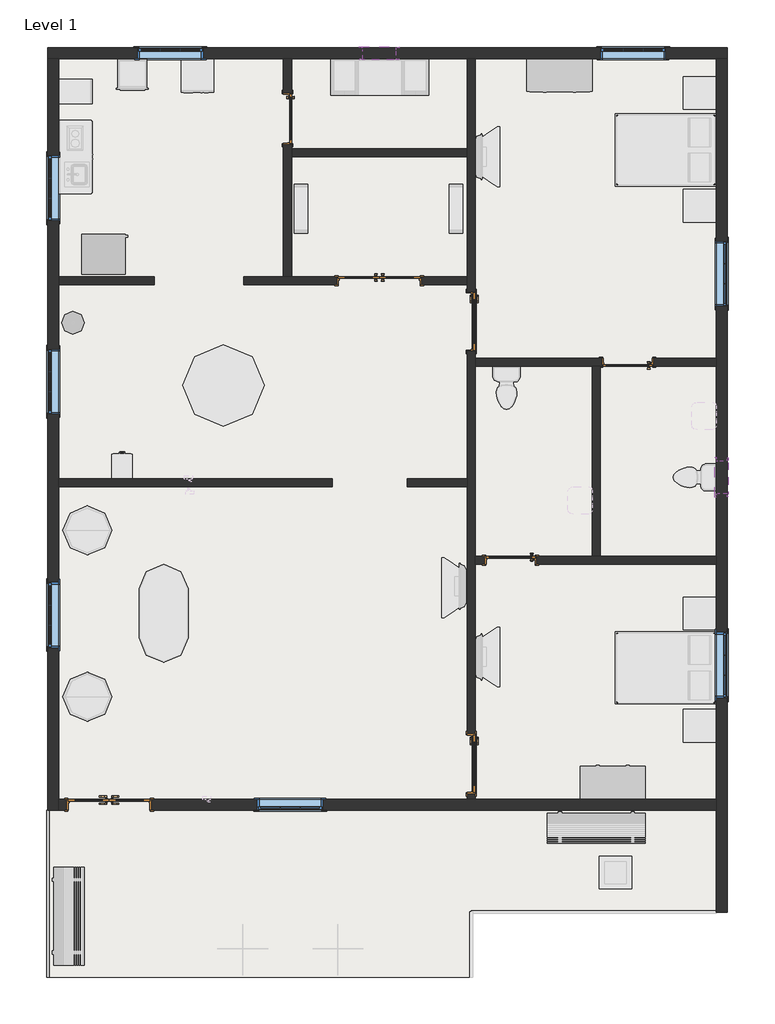
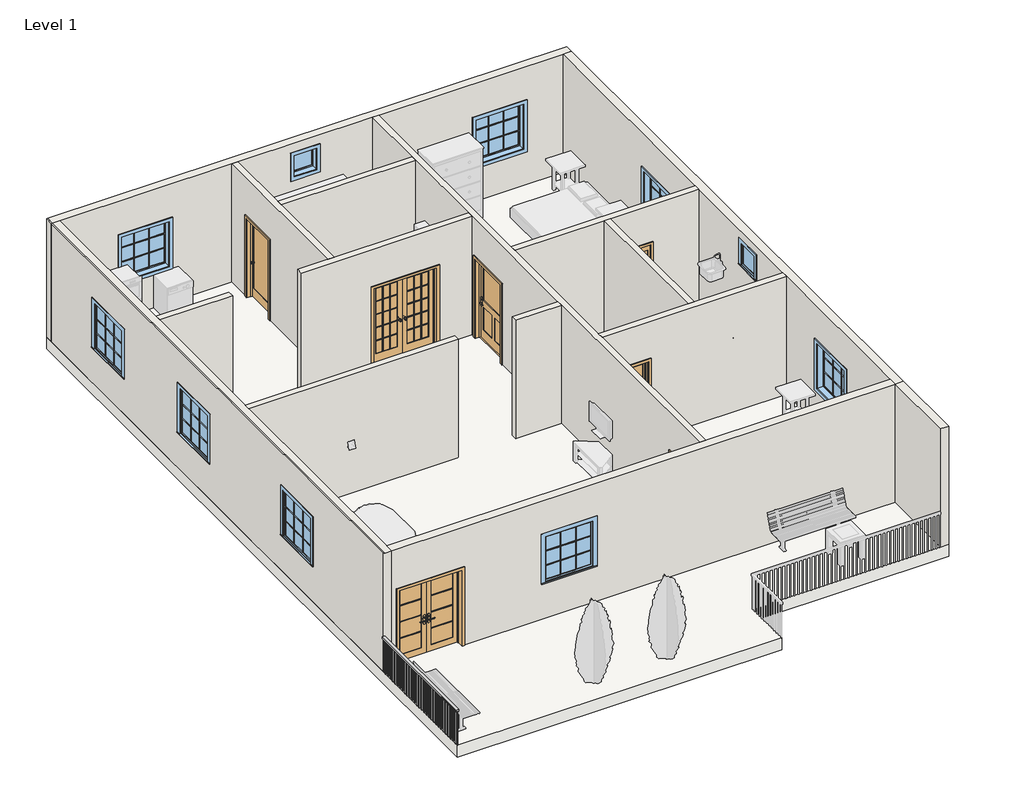
# One storey, part 1 of 2: 14 walls, 10 windows, 7 doors, 1 railing, 1 slab.
"""IFC4 building model written with IfcOpenShell, lengths in millimetres."""

from ifc_helpers import new_model, si_unit, frame, origin, origin_with_axes, place, context, project, spatial, polyline, outline, extrude, faceted_brep, transform, mapped, element, save
from components import door_f970b2d0, door_b03bd389, door_31a77bde, door_b28d7136, door_792ab218, window_791d807c, window_7418cbd4, window_e41d21a6

model = new_model("IFC4")

# Units and contexts
model_context = context("Model", 3, world=origin())
ifc_project = project(units=[si_unit("LENGTHUNIT", "METRE", prefix="MILLI")], contexts=[model_context])

# Site, building, storey
site = spatial("IfcSite", under=ifc_project)
building = spatial("IfcBuilding", under=site)
storey = spatial("IfcBuildingStorey", under=building, Name="Level 1", Elevation=0.0)

# Doors
placement = place(None, origin())
door_shape = door_f970b2d0(model_context)
element("IfcDoor", 1, ObjectType="30\" x 80\"", at=placement, inside=storey, context=model_context, shape_type="MappedRepresentation", body=[
    mapped(door_shape, transform((-7653.2898609, 8737.7801051, 0.0), x_axis=(0.0, 1.0, 0.0), y_axis=(-1.0, 0.0, 0.0), z_axis=(0.0, 0.0, 1.0))),
])
element("IfcDoor", 2, ObjectType="30\" x 80\"", at=placement, inside=storey, context=model_context, shape_type="MappedRepresentation", body=[
    mapped(door_shape, transform((-7653.2898609, 482.7801051, 0.0), x_axis=(0.0, 1.0, 0.0), y_axis=(-1.0, 0.0, 0.0), z_axis=(0.0, 0.0, 1.0))),
])
door_2_shape = door_b03bd389(model_context)
element("IfcDoor", 3, ObjectType="Door-Exterior-Double-Full Glass-Wood_Clad : 60\" x 80\"", at=placement, inside=storey, context=model_context, shape_type="MappedRepresentation", body=[
    mapped(door_2_shape, transform((-14412.8648609, -276.0448949, -76.2), x_axis=(1.0, 0.0, 0.0), y_axis=(0.0, 1.0, 0.0), z_axis=(0.0, 0.0, 1.0))),
])
door_3_shape = door_31a77bde(model_context)
element("IfcDoor", 4, ObjectType="Door-Interior-Double-Full Glass-Wood : 60\" x 80\"", at=placement, inside=storey, context=model_context, shape_type="MappedRepresentation", body=[
    mapped(door_3_shape, transform((-9370.9648609, 9502.9551051, 0.0), x_axis=(1.0, 0.0, 0.0), y_axis=(0.0, 1.0, 0.0), z_axis=(0.0, 0.0, 1.0))),
])
door_4_shape = door_b28d7136(model_context)
element("IfcDoor", 5, ObjectType="Door-Interior-Single-1_Panel-Wood : 12\" x 80\"", at=placement, inside=storey, context=model_context, shape_type="MappedRepresentation", body=[
    mapped(door_4_shape, transform((-4735.4648609, 7972.6051051, 0.0), x_axis=(-1.0, 0.0, 0.0), y_axis=(0.0, -1.0, 0.0), z_axis=(0.0, 0.0, 1.0))),
])
element("IfcDoor", 6, ObjectType="Door-Interior-Single-1_Panel-Wood : 12\" x 80\"", at=placement, inside=storey, context=model_context, shape_type="MappedRepresentation", body=[
    mapped(door_4_shape, transform((-11082.2898609, 12522.3801051, 0.0), x_axis=(0.0, -1.0, 0.0), y_axis=(1.0, 0.0, 0.0), z_axis=(0.0, 0.0, 1.0))),
])
door_5_shape = door_792ab218(model_context)
element("IfcDoor", 7, ObjectType="Door-Interior-Single-1_Panel-Wood : 12\" x 80\"", at=placement, inside=storey, context=model_context, shape_type="MappedRepresentation", body=[
    mapped(door_5_shape, transform((-6919.8648609, 4283.2551051, 0.0), x_axis=(-1.0, 0.0, 0.0), y_axis=(0.0, -1.0, 0.0), z_axis=(0.0, 0.0, 1.0))),
])

# Railing
element("IfcRailing", 8, ObjectType="Handrail - Rectangular", at=placement, inside=storey, context=model_context, shape_type="SweptSolid", body=[
    extrude(outline(polyline([(-15581.2648609, -380.8198949), (-15530.4648609, -380.8198949), (-15530.4648609, -3505.0198949), (-15581.2648609, -3505.0198949), (-15581.2648609, -380.8198949)])), frame((0.0, 0.0, 863.6), z_axis=(0.0, 0.0, 1.0), x_axis=(1.0, 0.0, 0.0)), (0.0, 0.0, 1.0), 50.8),
    extrude(outline(polyline([(-15565.3898609, -3419.2948949), (-15546.3398609, -3419.2948949), (-15546.3398609, -3438.3448949), (-15565.3898609, -3438.3448949), (-15565.3898609, -3419.2948949)])), origin_with_axes(), (0.0, 0.0, 1.0), 863.6),
    extrude(outline(polyline([(-15565.3898609, -3317.6948949), (-15546.3398609, -3317.6948949), (-15546.3398609, -3336.7448949), (-15565.3898609, -3336.7448949), (-15565.3898609, -3317.6948949)])), origin_with_axes(), (0.0, 0.0, 1.0), 863.6),
    extrude(outline(polyline([(-15565.3898609, -3216.0948949), (-15546.3398609, -3216.0948949), (-15546.3398609, -3235.1448949), (-15565.3898609, -3235.1448949), (-15565.3898609, -3216.0948949)])), origin_with_axes(), (0.0, 0.0, 1.0), 863.6),
    extrude(outline(polyline([(-15565.3898609, -3114.4948949), (-15546.3398609, -3114.4948949), (-15546.3398609, -3133.5448949), (-15565.3898609, -3133.5448949), (-15565.3898609, -3114.4948949)])), origin_with_axes(), (0.0, 0.0, 1.0), 863.6),
    extrude(outline(polyline([(-15565.3898609, -3012.8948949), (-15546.3398609, -3012.8948949), (-15546.3398609, -3031.9448949), (-15565.3898609, -3031.9448949), (-15565.3898609, -3012.8948949)])), origin_with_axes(), (0.0, 0.0, 1.0), 863.6),
    extrude(outline(polyline([(-15565.3898609, -2911.2948949), (-15546.3398609, -2911.2948949), (-15546.3398609, -2930.3448949), (-15565.3898609, -2930.3448949), (-15565.3898609, -2911.2948949)])), origin_with_axes(), (0.0, 0.0, 1.0), 863.6),
    extrude(outline(polyline([(-15565.3898609, -2809.6948949), (-15546.3398609, -2809.6948949), (-15546.3398609, -2828.7448949), (-15565.3898609, -2828.7448949), (-15565.3898609, -2809.6948949)])), origin_with_axes(), (0.0, 0.0, 1.0), 863.6),
    extrude(outline(polyline([(-15565.3898609, -2708.0948949), (-15546.3398609, -2708.0948949), (-15546.3398609, -2727.1448949), (-15565.3898609, -2727.1448949), (-15565.3898609, -2708.0948949)])), origin_with_axes(), (0.0, 0.0, 1.0), 863.6),
    extrude(outline(polyline([(-15565.3898609, -2606.4948949), (-15546.3398609, -2606.4948949), (-15546.3398609, -2625.5448949), (-15565.3898609, -2625.5448949), (-15565.3898609, -2606.4948949)])), origin_with_axes(), (0.0, 0.0, 1.0), 863.6),
    extrude(outline(polyline([(-15565.3898609, -2504.8948949), (-15546.3398609, -2504.8948949), (-15546.3398609, -2523.9448949), (-15565.3898609, -2523.9448949), (-15565.3898609, -2504.8948949)])), origin_with_axes(), (0.0, 0.0, 1.0), 863.6),
    extrude(outline(polyline([(-15565.3898609, -2403.2948949), (-15546.3398609, -2403.2948949), (-15546.3398609, -2422.3448949), (-15565.3898609, -2422.3448949), (-15565.3898609, -2403.2948949)])), origin_with_axes(), (0.0, 0.0, 1.0), 863.6),
    extrude(outline(polyline([(-15565.3898609, -2301.6948949), (-15546.3398609, -2301.6948949), (-15546.3398609, -2320.7448949), (-15565.3898609, -2320.7448949), (-15565.3898609, -2301.6948949)])), origin_with_axes(), (0.0, 0.0, 1.0), 863.6),
    extrude(outline(polyline([(-15565.3898609, -2200.0948949), (-15546.3398609, -2200.0948949), (-15546.3398609, -2219.1448949), (-15565.3898609, -2219.1448949), (-15565.3898609, -2200.0948949)])), origin_with_axes(), (0.0, 0.0, 1.0), 863.6),
    extrude(outline(polyline([(-15565.3898609, -2098.4948949), (-15546.3398609, -2098.4948949), (-15546.3398609, -2117.5448949), (-15565.3898609, -2117.5448949), (-15565.3898609, -2098.4948949)])), origin_with_axes(), (0.0, 0.0, 1.0), 863.6),
    extrude(outline(polyline([(-15565.3898609, -1996.8948949), (-15546.3398609, -1996.8948949), (-15546.3398609, -2015.9448949), (-15565.3898609, -2015.9448949), (-15565.3898609, -1996.8948949)])), origin_with_axes(), (0.0, 0.0, 1.0), 863.6),
    extrude(outline(polyline([(-15565.3898609, -1895.2948949), (-15546.3398609, -1895.2948949), (-15546.3398609, -1914.3448949), (-15565.3898609, -1914.3448949), (-15565.3898609, -1895.2948949)])), origin_with_axes(), (0.0, 0.0, 1.0), 863.6),
    extrude(outline(polyline([(-15565.3898609, -1793.6948949), (-15546.3398609, -1793.6948949), (-15546.3398609, -1812.7448949), (-15565.3898609, -1812.7448949), (-15565.3898609, -1793.6948949)])), origin_with_axes(), (0.0, 0.0, 1.0), 863.6),
    extrude(outline(polyline([(-15565.3898609, -1692.0948949), (-15546.3398609, -1692.0948949), (-15546.3398609, -1711.1448949), (-15565.3898609, -1711.1448949), (-15565.3898609, -1692.0948949)])), origin_with_axes(), (0.0, 0.0, 1.0), 863.6),
    extrude(outline(polyline([(-15565.3898609, -1590.4948949), (-15546.3398609, -1590.4948949), (-15546.3398609, -1609.5448949), (-15565.3898609, -1609.5448949), (-15565.3898609, -1590.4948949)])), origin_with_axes(), (0.0, 0.0, 1.0), 863.6),
    extrude(outline(polyline([(-15565.3898609, -1488.8948949), (-15546.3398609, -1488.8948949), (-15546.3398609, -1507.9448949), (-15565.3898609, -1507.9448949), (-15565.3898609, -1488.8948949)])), origin_with_axes(), (0.0, 0.0, 1.0), 863.6),
    extrude(outline(polyline([(-15565.3898609, -1387.2948949), (-15546.3398609, -1387.2948949), (-15546.3398609, -1406.3448949), (-15565.3898609, -1406.3448949), (-15565.3898609, -1387.2948949)])), origin_with_axes(), (0.0, 0.0, 1.0), 863.6),
    extrude(outline(polyline([(-15565.3898609, -1285.6948949), (-15546.3398609, -1285.6948949), (-15546.3398609, -1304.7448949), (-15565.3898609, -1304.7448949), (-15565.3898609, -1285.6948949)])), origin_with_axes(), (0.0, 0.0, 1.0), 863.6),
    extrude(outline(polyline([(-15565.3898609, -1184.0948949), (-15546.3398609, -1184.0948949), (-15546.3398609, -1203.1448949), (-15565.3898609, -1203.1448949), (-15565.3898609, -1184.0948949)])), origin_with_axes(), (0.0, 0.0, 1.0), 863.6),
    extrude(outline(polyline([(-15565.3898609, -1082.4948949), (-15546.3398609, -1082.4948949), (-15546.3398609, -1101.5448949), (-15565.3898609, -1101.5448949), (-15565.3898609, -1082.4948949)])), origin_with_axes(), (0.0, 0.0, 1.0), 863.6),
    extrude(outline(polyline([(-15565.3898609, -980.8948949), (-15546.3398609, -980.8948949), (-15546.3398609, -999.9448949), (-15565.3898609, -999.9448949), (-15565.3898609, -980.8948949)])), origin_with_axes(), (0.0, 0.0, 1.0), 863.6),
    extrude(outline(polyline([(-15565.3898609, -879.2948949), (-15546.3398609, -879.2948949), (-15546.3398609, -898.3448949), (-15565.3898609, -898.3448949), (-15565.3898609, -879.2948949)])), origin_with_axes(), (0.0, 0.0, 1.0), 863.6),
    extrude(outline(polyline([(-15565.3898609, -777.6948949), (-15546.3398609, -777.6948949), (-15546.3398609, -796.7448949), (-15565.3898609, -796.7448949), (-15565.3898609, -777.6948949)])), origin_with_axes(), (0.0, 0.0, 1.0), 863.6),
    extrude(outline(polyline([(-15565.3898609, -676.0948949), (-15546.3398609, -676.0948949), (-15546.3398609, -695.1448949), (-15565.3898609, -695.1448949), (-15565.3898609, -676.0948949)])), origin_with_axes(), (0.0, 0.0, 1.0), 863.6),
    extrude(outline(polyline([(-15565.3898609, -574.4948949), (-15546.3398609, -574.4948949), (-15546.3398609, -593.5448949), (-15565.3898609, -593.5448949), (-15565.3898609, -574.4948949)])), origin_with_axes(), (0.0, 0.0, 1.0), 863.6),
    extrude(outline(polyline([(-15565.3898609, -472.8948949), (-15546.3398609, -472.8948949), (-15546.3398609, -491.9448949), (-15565.3898609, -491.9448949), (-15565.3898609, -472.8948949)])), origin_with_axes(), (0.0, 0.0, 1.0), 863.6),
    extrude(outline(polyline([(-15565.3898609, -3485.9698949), (-15546.3398609, -3485.9698949), (-15546.3398609, -3505.0198949), (-15565.3898609, -3505.0198949), (-15565.3898609, -3485.9698949)])), origin_with_axes(), (0.0, 0.0, 1.0), 863.6),
    extrude(outline(polyline([(-15565.3898609, -380.8198949), (-15546.3398609, -380.8198949), (-15546.3398609, -399.8698949), (-15565.3898609, -399.8698949), (-15565.3898609, -380.8198949)])), origin_with_axes(), (0.0, 0.0, 1.0), 863.6),
])

# Slab
element("IfcSlab", 9, ObjectType="Generic - 12\"", at=placement, inside=storey, context=model_context, shape_type="SweptSolid", body=[
    extrude(outline(polyline([(-2881.2648609, 13843.1801051), (-2881.2648609, -2285.8198949), (-7656.4648609, -2285.8198949), (-7656.4648609, -3505.0198949), (-15555.8648609, -3505.0198949), (-15555.8648609, 13843.1801051), (-2881.2648609, 13843.1801051)])), frame((0.0, 0.0, -304.8), z_axis=(0.0, 0.0, 1.0), x_axis=(1.0, 0.0, 0.0)), (0.0, 0.0, 1.0), 304.8),
])

# Walls
element("IfcWall", 10, ObjectType="Generic - 8\"", at=placement, inside=storey, context=model_context, shape_type="Brep", body=[
    faceted_brep([(-15555.8648609, 13639.9801051, 0.0), (-15352.6648609, 13639.9801051, 0.0), (-11161.6648609, 13639.9801051, 0.0), (-11009.2648609, 13639.9801051, 0.0), (-7732.6648609, 13639.9801051, 0.0), (-7580.2648609, 13639.9801051, 0.0), (-3084.4648609, 13639.9801051, 0.0), (-2881.2648609, 13639.9801051, 0.0), (-2881.2648609, 13639.9801051, 3048.0), (-3084.4648609, 13639.9801051, 3048.0), (-7580.2648609, 13639.9801051, 3048.0), (-7732.6648609, 13639.9801051, 3048.0), (-11009.2648609, 13639.9801051, 3048.0), (-11161.6648609, 13639.9801051, 3048.0), (-15352.6648609, 13639.9801051, 3048.0), (-15530.4648609, 13639.9801051, 3048.0), (-15555.8648609, 13639.9801051, 3048.0), (-4024.2648609, 13639.9801051, 2133.6), (-4024.2648609, 13639.9801051, 914.4), (-5243.4648609, 13639.9801051, 914.4), (-5243.4648609, 13639.9801051, 2133.6), (-12660.2648609, 13639.9801051, 2133.6), (-12660.2648609, 13639.9801051, 914.4), (-13879.4648609, 13639.9801051, 914.4), (-13879.4648609, 13639.9801051, 2133.6), (-9066.1648609, 13639.9801051, 2768.6), (-9066.1648609, 13639.9801051, 2159.0), (-9675.7648609, 13639.9801051, 2159.0), (-9675.7648609, 13639.9801051, 2768.6), (-15555.8648609, 13843.1801051, 0.0), (-15555.8648609, 13843.1801051, 3048.0), (-15530.4648609, 13843.1801051, 3048.0), (-2881.2648609, 13843.1801051, 3048.0), (-2881.2648609, 13843.1801051, 0.0), (-4024.2648609, 13843.1801051, 2133.6), (-5243.4648609, 13843.1801051, 2133.6), (-5243.4648609, 13843.1801051, 914.4), (-4024.2648609, 13843.1801051, 914.4), (-12660.2648609, 13843.1801051, 2133.6), (-13879.4648609, 13843.1801051, 2133.6), (-13879.4648609, 13843.1801051, 914.4), (-12660.2648609, 13843.1801051, 914.4), (-9066.1648609, 13843.1801051, 2768.6), (-9675.7648609, 13843.1801051, 2768.6), (-9675.7648609, 13843.1801051, 2159.0), (-9066.1648609, 13843.1801051, 2159.0)], [[[0, 1, 2, 3, 4, 5, 6, 7, 8, 9, 10, 11, 12, 13, 14, 15, 16], [17, 18, 19, 20], [21, 22, 23, 24], [25, 26, 27, 28]], [[29, 30, 31, 32, 33], [34, 35, 36, 37], [38, 39, 40, 41], [42, 43, 44, 45]], [[7, 6, 5, 4, 3, 2, 1, 0, 29, 33]], [[8, 7, 33, 32]], [[0, 16, 30, 29]], [[18, 17, 34, 37]], [[19, 18, 37, 36]], [[20, 19, 36, 35]], [[17, 20, 35, 34]], [[22, 21, 38, 41]], [[23, 22, 41, 40]], [[24, 23, 40, 39]], [[21, 24, 39, 38]], [[26, 25, 42, 45]], [[27, 26, 45, 44]], [[28, 27, 44, 43]], [[25, 28, 43, 42]], [[16, 15, 31, 30]], [[15, 14, 13, 12, 11, 10, 9, 8, 32, 31]]]),
])
element("IfcWall", 11, ObjectType="Generic - 8\"", at=placement, inside=storey, context=model_context, shape_type="Brep", body=[
    faceted_brep([(-3084.4648609, 13639.9801051, 0.0), (-3084.4648609, 8051.9801051, 0.0), (-3084.4648609, 7899.5801051, 0.0), (-3084.4648609, 4356.2801051, 0.0), (-3084.4648609, 4203.8801051, 0.0), (-3084.4648609, -177.6198949, 0.0), (-3084.4648609, -380.8198949, 0.0), (-3084.4648609, -2285.8198949, 0.0), (-3084.4648609, -2285.8198949, 3048.0), (-3084.4648609, -380.8198949, 3048.0), (-3084.4648609, -177.6198949, 3048.0), (-3084.4648609, 4203.8801051, 3048.0), (-3084.4648609, 4356.2801051, 3048.0), (-3084.4648609, 7899.5801051, 3048.0), (-3084.4648609, 8051.9801051, 3048.0), (-3084.4648609, 13639.9801051, 3048.0), (-3084.4648609, 1714.6801051, 2133.6), (-3084.4648609, 1714.6801051, 914.4), (-3084.4648609, 2933.8801051, 914.4), (-3084.4648609, 2933.8801051, 2133.6), (-3084.4648609, 9017.1801051, 2133.6), (-3084.4648609, 9017.1801051, 914.4), (-3084.4648609, 10236.3801051, 914.4), (-3084.4648609, 10236.3801051, 2133.6), (-3084.4648609, 6134.2801051, 2768.6), (-3084.4648609, 5524.6801051, 2768.6), (-3084.4648609, 5524.6801051, 2159.0), (-3084.4648609, 6134.2801051, 2159.0), (-2881.2648609, 13639.9801051, 0.0), (-2881.2648609, 13639.9801051, 3048.0), (-2881.2648609, -380.8198949, 3048.0), (-2881.2648609, -2285.8198949, 3048.0), (-2881.2648609, -2285.8198949, 0.0), (-2881.2648609, 1714.6801051, 2133.6), (-2881.2648609, 2933.8801051, 2133.6), (-2881.2648609, 2933.8801051, 914.4), (-2881.2648609, 1714.6801051, 914.4), (-2881.2648609, 9017.1801051, 2133.6), (-2881.2648609, 10236.3801051, 2133.6), (-2881.2648609, 10236.3801051, 914.4), (-2881.2648609, 9017.1801051, 914.4), (-2881.2648609, 6134.2801051, 2768.6), (-2881.2648609, 6134.2801051, 2159.0), (-2881.2648609, 5524.6801051, 2159.0), (-2881.2648609, 5524.6801051, 2768.6)], [[[0, 1, 2, 3, 4, 5, 6, 7, 8, 9, 10, 11, 12, 13, 14, 15], [16, 17, 18, 19], [20, 21, 22, 23], [24, 25, 26, 27]], [[28, 29, 30, 31, 32], [33, 34, 35, 36], [37, 38, 39, 40], [41, 42, 43, 44]], [[7, 6, 5, 4, 3, 2, 1, 0, 28, 32]], [[8, 7, 32, 31]], [[0, 15, 29, 28]], [[17, 16, 33, 36]], [[18, 17, 36, 35]], [[19, 18, 35, 34]], [[16, 19, 34, 33]], [[21, 20, 37, 40]], [[22, 21, 40, 39]], [[23, 22, 39, 38]], [[20, 23, 38, 37]], [[42, 41, 24, 27]], [[43, 42, 27, 26]], [[44, 43, 26, 25]], [[41, 44, 25, 24]], [[9, 8, 31, 30]], [[15, 14, 13, 12, 11, 10, 9, 30, 29]]]),
])
element("IfcWall", 12, ObjectType="Generic - 8\"", at=placement, inside=storey, context=model_context, shape_type="Brep", body=[
    faceted_brep([(-3084.4648609, -177.6198949, 3048.0), (-3084.4648609, -177.6198949, 0.0), (-7580.2648609, -177.6198949, 0.0), (-7732.6648609, -177.6198949, 0.0), (-13625.4648609, -177.6198949, 0.0), (-13625.4648609, -177.6198949, 1981.2), (-15200.2648609, -177.6198949, 1981.2), (-15200.2648609, -177.6198949, 0.0), (-15352.6648609, -177.6198949, 0.0), (-15352.6648609, -177.6198949, 3048.0), (-7732.6648609, -177.6198949, 3048.0), (-7580.2648609, -177.6198949, 3048.0), (-10425.0648609, -177.6198949, 2133.6), (-11644.2648609, -177.6198949, 2133.6), (-11644.2648609, -177.6198949, 914.4), (-10425.0648609, -177.6198949, 914.4), (-3084.4648609, -380.8198949, 0.0), (-3084.4648609, -380.8198949, 3048.0), (-15352.6648609, -380.8198949, 3048.0), (-15352.6648609, -380.8198949, 0.0), (-15200.2648609, -380.8198949, 0.0), (-15200.2648609, -380.8198949, 1981.2), (-13625.4648609, -380.8198949, 1981.2), (-13625.4648609, -380.8198949, 0.0), (-10425.0648609, -380.8198949, 2133.6), (-10425.0648609, -380.8198949, 914.4), (-11644.2648609, -380.8198949, 914.4), (-11644.2648609, -380.8198949, 2133.6)], [[[0, 1, 2, 3, 4, 5, 6, 7, 8, 9, 10, 11], [12, 13, 14, 15]], [[16, 17, 18, 19, 20, 21, 22, 23], [24, 25, 26, 27]], [[1, 16, 23, 4, 3, 2]], [[19, 8, 7, 20]], [[1, 0, 17, 16]], [[9, 8, 19, 18]], [[22, 5, 4, 23]], [[5, 22, 21, 6]], [[6, 21, 20, 7]], [[25, 24, 12, 15]], [[26, 25, 15, 14]], [[27, 26, 14, 13]], [[24, 27, 13, 12]], [[0, 11, 10, 9, 18, 17]]]),
])
element("IfcWall", 13, ObjectType="Generic - 8\"", at=placement, inside=storey, context=model_context, shape_type="Brep", body=[
    faceted_brep([(-15352.6648609, -380.8198949, 0.0), (-15352.6648609, -177.6198949, 0.0), (-15352.6648609, 5651.6801051, 0.0), (-15352.6648609, 5804.0801051, 0.0), (-15352.6648609, 9423.5801051, 0.0), (-15352.6648609, 9575.9801051, 0.0), (-15352.6648609, 13639.9801051, 0.0), (-15352.6648609, 13639.9801051, 3048.0), (-15352.6648609, 9575.9801051, 3048.0), (-15352.6648609, 9423.5801051, 3048.0), (-15352.6648609, 5804.0801051, 3048.0), (-15352.6648609, 5651.6801051, 3048.0), (-15352.6648609, -177.6198949, 3048.0), (-15352.6648609, -380.8198949, 3048.0), (-15352.6648609, 11836.5801051, 2133.6), (-15352.6648609, 11836.5801051, 914.4), (-15352.6648609, 10617.3801051, 914.4), (-15352.6648609, 10617.3801051, 2133.6), (-15352.6648609, 8223.4301051, 2133.6), (-15352.6648609, 8223.4301051, 914.4), (-15352.6648609, 7004.2301051, 914.4), (-15352.6648609, 7004.2301051, 2133.6), (-15352.6648609, 3867.3301051, 2133.6), (-15352.6648609, 3867.3301051, 914.4), (-15352.6648609, 2648.1301051, 914.4), (-15352.6648609, 2648.1301051, 2133.6), (-15555.8648609, -380.8198949, 0.0), (-15555.8648609, -380.8198949, 3048.0), (-15555.8648609, 13639.9801051, 3048.0), (-15555.8648609, 13639.9801051, 0.0), (-15555.8648609, 11836.5801051, 2133.6), (-15555.8648609, 10617.3801051, 2133.6), (-15555.8648609, 10617.3801051, 914.4), (-15555.8648609, 11836.5801051, 914.4), (-15555.8648609, 8223.4301051, 2133.6), (-15555.8648609, 7004.2301051, 2133.6), (-15555.8648609, 7004.2301051, 914.4), (-15555.8648609, 8223.4301051, 914.4), (-15555.8648609, 3867.3301051, 2133.6), (-15555.8648609, 2648.1301051, 2133.6), (-15555.8648609, 2648.1301051, 914.4), (-15555.8648609, 3867.3301051, 914.4), (-15530.4648609, 13639.9801051, 3048.0), (-15530.4648609, -380.8198949, 3048.0)], [[[0, 1, 2, 3, 4, 5, 6, 7, 8, 9, 10, 11, 12, 13], [14, 15, 16, 17], [18, 19, 20, 21], [22, 23, 24, 25]], [[26, 27, 28, 29], [30, 31, 32, 33], [34, 35, 36, 37], [38, 39, 40, 41]], [[6, 5, 4, 3, 2, 1, 0, 26, 29]], [[7, 6, 29, 28, 42]], [[0, 13, 43, 27, 26]], [[15, 14, 30, 33]], [[16, 15, 33, 32]], [[17, 16, 32, 31]], [[14, 17, 31, 30]], [[19, 18, 34, 37]], [[20, 19, 37, 36]], [[21, 20, 36, 35]], [[18, 21, 35, 34]], [[23, 22, 38, 41]], [[24, 23, 41, 40]], [[25, 24, 40, 39]], [[22, 25, 39, 38]], [[42, 28, 27, 43]], [[13, 12, 11, 10, 9, 8, 7, 42, 43]]]),
])
element("IfcWall", 14, ObjectType="INNER WALL", at=placement, inside=storey, context=model_context, shape_type="Brep", body=[
    faceted_brep([(-7732.6648609, 13639.9801051, 3048.0), (-7732.6648609, 13639.9801051, 0.0), (-7732.6648609, 11963.5801051, 0.0), (-7732.6648609, 11811.1801051, 0.0), (-7732.6648609, 9575.9801051, 0.0), (-7732.6648609, 9423.5801051, 0.0), (-7732.6648609, 9296.5801051, 0.0), (-7732.6648609, 9296.5801051, 2057.4), (-7732.6648609, 8178.9801051, 2057.4), (-7732.6648609, 8178.9801051, 0.0), (-7732.6648609, 5804.0801051, 0.0), (-7732.6648609, 5651.6801051, 0.0), (-7732.6648609, 1041.5801051, 0.0), (-7732.6648609, 1041.5801051, 2057.4), (-7732.6648609, -76.0198949, 2057.4), (-7732.6648609, -76.0198949, 0.0), (-7732.6648609, -177.6198949, 0.0), (-7732.6648609, -177.6198949, 3048.0), (-7732.6648609, 5651.6801051, 3048.0), (-7732.6648609, 5804.0801051, 3048.0), (-7732.6648609, 9423.5801051, 3048.0), (-7732.6648609, 9575.9801051, 3048.0), (-7732.6648609, 11811.1801051, 3048.0), (-7732.6648609, 11963.5801051, 3048.0), (-7580.2648609, 13639.9801051, 0.0), (-7580.2648609, 13639.9801051, 3048.0), (-7580.2648609, 8051.9801051, 3048.0), (-7580.2648609, 7899.5801051, 3048.0), (-7580.2648609, 4356.2801051, 3048.0), (-7580.2648609, 4203.8801051, 3048.0), (-7580.2648609, -177.6198949, 3048.0), (-7580.2648609, -177.6198949, 0.0), (-7580.2648609, -76.0198949, 0.0), (-7580.2648609, -76.0198949, 2057.4), (-7580.2648609, 1041.5801051, 2057.4), (-7580.2648609, 1041.5801051, 0.0), (-7580.2648609, 4203.8801051, 0.0), (-7580.2648609, 4356.2801051, 0.0), (-7580.2648609, 7899.5801051, 0.0), (-7580.2648609, 8051.9801051, 0.0), (-7580.2648609, 8178.9801051, 0.0), (-7580.2648609, 8178.9801051, 2057.4), (-7580.2648609, 9296.5801051, 2057.4), (-7580.2648609, 9296.5801051, 0.0)], [[[0, 1, 2, 3, 4, 5, 6, 7, 8, 9, 10, 11, 12, 13, 14, 15, 16, 17, 18, 19, 20, 21, 22, 23]], [[24, 25, 26, 27, 28, 29, 30, 31, 32, 33, 34, 35, 36, 37, 38, 39, 40, 41, 42, 43]], [[1, 24, 43, 6, 5, 4, 3, 2]], [[31, 16, 15, 32]], [[9, 40, 39, 38, 37, 36, 35, 12, 11, 10]], [[1, 0, 25, 24]], [[17, 16, 31, 30]], [[42, 7, 6, 43]], [[7, 42, 41, 8]], [[8, 41, 40, 9]], [[34, 13, 12, 35]], [[13, 34, 33, 14]], [[14, 33, 32, 15]], [[0, 23, 22, 21, 20, 19, 18, 17, 30, 29, 28, 27, 26, 25]]]),
])
element("IfcWall", 15, ObjectType="INNER WALL", at=placement, inside=storey, context=model_context, shape_type="Brep", body=[
    faceted_brep([(-11161.6648609, 13639.9801051, 3048.0), (-11161.6648609, 13639.9801051, 0.0), (-11161.6648609, 13004.9801051, 0.0), (-11161.6648609, 13004.9801051, 2057.4), (-11161.6648609, 12039.7801051, 2057.4), (-11161.6648609, 12039.7801051, 0.0), (-11161.6648609, 9575.9801051, 0.0), (-11161.6648609, 9575.9801051, 3048.0), (-11009.2648609, 13639.9801051, 0.0), (-11009.2648609, 13639.9801051, 3048.0), (-11009.2648609, 11963.5801051, 3048.0), (-11009.2648609, 11811.1801051, 3048.0), (-11009.2648609, 9575.9801051, 3048.0), (-11009.2648609, 9575.9801051, 0.0), (-11009.2648609, 11811.1801051, 0.0), (-11009.2648609, 11963.5801051, 0.0), (-11009.2648609, 12039.7801051, 0.0), (-11009.2648609, 12039.7801051, 2057.4), (-11009.2648609, 13004.9801051, 2057.4), (-11009.2648609, 13004.9801051, 0.0)], [[[0, 1, 2, 3, 4, 5, 6, 7]], [[8, 9, 10, 11, 12, 13, 14, 15, 16, 17, 18, 19]], [[1, 8, 19, 2]], [[13, 6, 5, 16, 15, 14]], [[1, 0, 9, 8]], [[7, 6, 13, 12]], [[4, 17, 16, 5]], [[17, 4, 3, 18]], [[18, 3, 2, 19]], [[0, 7, 12, 11, 10, 9]]]),
])
element("IfcWall", 16, ObjectType="INNER WALL", at=placement, inside=storey, context=model_context, shape_type="SweptSolid", body=[
    extrude(outline(polyline([(-13574.6648609, 9423.5801051), (-15352.6648609, 9423.5801051), (-15352.6648609, 9575.9801051), (-13574.6648609, 9575.9801051), (-13574.6648609, 9423.5801051)])), origin_with_axes(), (0.0, 0.0, 1.0), 3048.0),
])
element("IfcWall", 17, ObjectType="INNER WALL", at=placement, inside=storey, context=model_context, shape_type="SweptSolid", body=[
    extrude(outline(polyline([(-8850.2648609, 5804.0801051), (-7732.6648609, 5804.0801051), (-7732.6648609, 5651.6801051), (-8850.2648609, 5651.6801051), (-8850.2648609, 5804.0801051)])), origin_with_axes(), (0.0, 0.0, 1.0), 3048.0),
])
element("IfcWall", 18, ObjectType="INNER WALL", at=placement, inside=storey, context=model_context, shape_type="Brep", body=[
    faceted_brep([(-3084.4648609, 7899.5801051, 0.0), (-3084.4648609, 7899.5801051, 3048.0), (-5243.4648609, 7899.5801051, 3048.0), (-5395.8648609, 7899.5801051, 3048.0), (-7580.2648609, 7899.5801051, 3048.0), (-7580.2648609, 7899.5801051, 0.0), (-5395.8648609, 7899.5801051, 0.0), (-5243.4648609, 7899.5801051, 0.0), (-5218.0648609, 7899.5801051, 0.0), (-5218.0648609, 7899.5801051, 2057.4), (-4252.8648609, 7899.5801051, 2057.4), (-4252.8648609, 7899.5801051, 0.0), (-3084.4648609, 8051.9801051, 3048.0), (-3084.4648609, 8051.9801051, 0.0), (-4252.8648609, 8051.9801051, 0.0), (-4252.8648609, 8051.9801051, 2057.4), (-5218.0648609, 8051.9801051, 2057.4), (-5218.0648609, 8051.9801051, 0.0), (-7580.2648609, 8051.9801051, 0.0), (-7580.2648609, 8051.9801051, 3048.0)], [[[0, 1, 2, 3, 4, 5, 6, 7, 8, 9, 10, 11]], [[12, 13, 14, 15, 16, 17, 18, 19]], [[5, 18, 17, 8, 7, 6]], [[13, 0, 11, 14]], [[1, 0, 13, 12]], [[5, 4, 19, 18]], [[16, 9, 8, 17]], [[9, 16, 15, 10]], [[10, 15, 14, 11]], [[4, 3, 2, 1, 12, 19]]]),
])
element("IfcWall", 19, ObjectType="INNER WALL", at=placement, inside=storey, context=model_context, shape_type="Brep", body=[
    faceted_brep([(-3084.4648609, 4356.2801051, 3048.0), (-3084.4648609, 4356.2801051, 0.0), (-5243.4648609, 4356.2801051, 0.0), (-5395.8648609, 4356.2801051, 0.0), (-6437.2648609, 4356.2801051, 0.0), (-6437.2648609, 4356.2801051, 2057.4), (-7402.4648609, 4356.2801051, 2057.4), (-7402.4648609, 4356.2801051, 0.0), (-7580.2648609, 4356.2801051, 0.0), (-7580.2648609, 4356.2801051, 3048.0), (-5395.8648609, 4356.2801051, 3048.0), (-5243.4648609, 4356.2801051, 3048.0), (-3084.4648609, 4203.8801051, 0.0), (-3084.4648609, 4203.8801051, 3048.0), (-7580.2648609, 4203.8801051, 3048.0), (-7580.2648609, 4203.8801051, 0.0), (-7402.4648609, 4203.8801051, 0.0), (-7402.4648609, 4203.8801051, 2057.4), (-6437.2648609, 4203.8801051, 2057.4), (-6437.2648609, 4203.8801051, 0.0)], [[[0, 1, 2, 3, 4, 5, 6, 7, 8, 9, 10, 11]], [[12, 13, 14, 15, 16, 17, 18, 19]], [[1, 12, 19, 4, 3, 2]], [[15, 8, 7, 16]], [[1, 0, 13, 12]], [[9, 8, 15, 14]], [[6, 17, 16, 7]], [[17, 6, 5, 18]], [[18, 5, 4, 19]], [[0, 11, 10, 9, 14, 13]]]),
])
element("IfcWall", 20, ObjectType="INNER WALL", at=placement, inside=storey, context=model_context, shape_type="SweptSolid", body=[
    extrude(outline(polyline([(-5395.8648609, 4356.2801051), (-5395.8648609, 7899.5801051), (-5243.4648609, 7899.5801051), (-5243.4648609, 4356.2801051), (-5395.8648609, 4356.2801051)])), origin_with_axes(), (0.0, 0.0, 1.0), 3048.0),
])
element("IfcWall", 21, ObjectType="INNER WALL", at=placement, inside=storey, context=model_context, shape_type="SweptSolid", body=[
    extrude(outline(polyline([(-11009.2648609, 11963.5801051), (-7732.6648609, 11963.5801051), (-7732.6648609, 11811.1801051), (-11009.2648609, 11811.1801051), (-11009.2648609, 11963.5801051)])), origin_with_axes(), (0.0, 0.0, 1.0), 3048.0),
])
element("IfcWall", 22, ObjectType="INNER WALL", at=placement, inside=storey, context=model_context, shape_type="SweptSolid", body=[
    extrude(outline(polyline([(-15352.6648609, 5804.0801051), (-10247.2648609, 5804.0801051), (-10247.2648609, 5651.6801051), (-15352.6648609, 5651.6801051), (-15352.6648609, 5804.0801051)])), origin_with_axes(), (0.0, 0.0, 1.0), 3048.0),
])
element("IfcWall", 23, ObjectType="INNER WALL", at=placement, inside=storey, context=model_context, shape_type="Brep", body=[
    faceted_brep([(-11898.2648609, 9423.5801051, 3048.0), (-11898.2648609, 9423.5801051, 0.0), (-10158.3648609, 9423.5801051, 0.0), (-10158.3648609, 9423.5801051, 2057.4), (-8583.5648609, 9423.5801051, 2057.4), (-8583.5648609, 9423.5801051, 0.0), (-7732.6648609, 9423.5801051, 0.0), (-7732.6648609, 9423.5801051, 3048.0), (-11898.2648609, 9575.9801051, 0.0), (-11898.2648609, 9575.9801051, 3048.0), (-11161.6648609, 9575.9801051, 3048.0), (-11009.2648609, 9575.9801051, 3048.0), (-7732.6648609, 9575.9801051, 3048.0), (-7732.6648609, 9575.9801051, 0.0), (-8583.5648609, 9575.9801051, 0.0), (-8583.5648609, 9575.9801051, 2057.4), (-10158.3648609, 9575.9801051, 2057.4), (-10158.3648609, 9575.9801051, 0.0), (-11009.2648609, 9575.9801051, 0.0), (-11161.6648609, 9575.9801051, 0.0)], [[[0, 1, 2, 3, 4, 5, 6, 7]], [[8, 9, 10, 11, 12, 13, 14, 15, 16, 17, 18, 19]], [[1, 8, 19, 18, 17, 2]], [[13, 6, 5, 14]], [[1, 0, 9, 8]], [[7, 6, 13, 12]], [[4, 15, 14, 5]], [[15, 4, 3, 16]], [[16, 3, 2, 17]], [[0, 7, 12, 11, 10, 9]]]),
])

# Windows
window_shape = window_791d807c(model_context)
element("IfcWindow", 24, ObjectType="Casement 3x3 with Trim : 36\" x 48\"", at=placement, inside=storey, context=model_context, shape_type="MappedRepresentation", body=[
    mapped(window_shape, transform((-11034.6648609, -279.2198949, 0.0), x_axis=(1.0, 0.0, 0.0), y_axis=(0.0, 1.0, 0.0), z_axis=(0.0, 0.0, 1.0))),
])
window_2_shape = window_7418cbd4(model_context)
element("IfcWindow", 25, ObjectType="Casement 3x3 with Trim : 36\" x 48\"", at=placement, inside=storey, context=model_context, shape_type="MappedRepresentation", body=[
    mapped(window_2_shape, transform((-2982.8648609, 2324.2801051, 0.0), x_axis=(0.0, -1.0, 0.0), y_axis=(1.0, 0.0, 0.0), z_axis=(0.0, 0.0, 1.0))),
])
element("IfcWindow", 26, ObjectType="Casement 3x3 with Trim : 36\" x 48\"", at=placement, inside=storey, context=model_context, shape_type="MappedRepresentation", body=[
    mapped(window_2_shape, transform((-2982.8648609, 9626.7801051, 0.0), x_axis=(0.0, -1.0, 0.0), y_axis=(1.0, 0.0, 0.0), z_axis=(0.0, 0.0, 1.0))),
])
element("IfcWindow", 27, ObjectType="Casement 3x3 with Trim : 36\" x 48\"", at=placement, inside=storey, context=model_context, shape_type="MappedRepresentation", body=[
    mapped(window_2_shape, transform((-4633.8648609, 13741.5801051, 0.0), x_axis=(1.0, 0.0, 0.0), y_axis=(0.0, 1.0, 0.0), z_axis=(0.0, 0.0, 1.0))),
])
element("IfcWindow", 28, ObjectType="Casement 3x3 with Trim : 36\" x 48\"", at=placement, inside=storey, context=model_context, shape_type="MappedRepresentation", body=[
    mapped(window_2_shape, transform((-13269.8648609, 13741.5801051, 0.0), x_axis=(1.0, 0.0, 0.0), y_axis=(0.0, 1.0, 0.0), z_axis=(0.0, 0.0, 1.0))),
])
element("IfcWindow", 29, ObjectType="Casement 3x3 with Trim : 36\" x 48\"", at=placement, inside=storey, context=model_context, shape_type="MappedRepresentation", body=[
    mapped(window_2_shape, transform((-15454.2648609, 11226.9801051, 0.0), x_axis=(0.0, 1.0, 0.0), y_axis=(-1.0, 0.0, 0.0), z_axis=(0.0, 0.0, 1.0))),
])
element("IfcWindow", 30, ObjectType="Casement 3x3 with Trim : 36\" x 48\"", at=placement, inside=storey, context=model_context, shape_type="MappedRepresentation", body=[
    mapped(window_2_shape, transform((-15454.2648609, 7613.8301051, 0.0), x_axis=(0.0, 1.0, 0.0), y_axis=(-1.0, 0.0, 0.0), z_axis=(0.0, 0.0, 1.0))),
])
element("IfcWindow", 31, ObjectType="Casement 3x3 with Trim : 36\" x 48\"", at=placement, inside=storey, context=model_context, shape_type="MappedRepresentation", body=[
    mapped(window_2_shape, transform((-15454.2648609, 3257.7301051, 0.0), x_axis=(0.0, 1.0, 0.0), y_axis=(-1.0, 0.0, 0.0), z_axis=(0.0, 0.0, 1.0))),
])
window_3_shape = window_e41d21a6(model_context)
element("IfcWindow", 32, ObjectType="Transom with Trim : 24\" x 24\"", at=placement, inside=storey, context=model_context, shape_type="MappedRepresentation", body=[
    mapped(window_3_shape, transform((-2982.8648609, 5867.5801051, 0.0), x_axis=(0.0, 1.0, 0.0), y_axis=(-1.0, 0.0, 0.0), z_axis=(0.0, 0.0, 1.0))),
])
element("IfcWindow", 33, ObjectType="Transom with Trim : 24\" x 24\"", at=placement, inside=storey, context=model_context, shape_type="MappedRepresentation", body=[
    mapped(window_3_shape, transform((-9332.8648609, 13741.5801051, 0.0), x_axis=(1.0, 0.0, 0.0), y_axis=(0.0, 1.0, 0.0), z_axis=(0.0, 0.0, 1.0))),
])

save(model, "model.ifc")

# Revit data of these elements
# Type "30\" x 80\""
#   Type Mark = "11"
#   Assembly Code = "B2030100"
#   Analytic Construction = "French door, wood frame with single glass"
#   Top Rail = 0' - 4 3/4"
#   Threshold Offset [instance default] = 0' - 0 1/2"
#   Thickness = 0' - 1 3/8"
#   Thermal Resistance (R) = 1.0696 (h·ft²·°F)/BTU
#   Swing Angle [instance default] = 90.00°
#   Stiles = 0' - 4 3/4"
#   Rough Width = 3' - 8"
#   Rough Height = 6' - 9"
#   Lock Rail = 0' - 7 1/8"
#   Height = 6' - 8"
#   Width = 3' - 6"
#   Heat Transfer Coefficient (U) = 0.9350 BTU/(h·ft²·°F)
#   Door Offset [instance default] = 0' - 0"
#   Bottom Rail = 0' - 9 1/2"
#   Threshold [instance default] = yes
#   Function = 1
#   Exterior Trim [instance default] = yes
#   Trim Material = Cherry
#   Threshold Material = Cherry
#   Panel Material = Cherry
#   Glazing = Glass
#   Frame Material = Cherry
#   Door Handle Material = Aluminum
#   Visual Light Transmittance = 0
#   Solar Heat Gain Coefficient = 0
#   Wall Closure = (empty or 0)
#   Construction Type = (empty or 0)
# Type "Door-Exterior-Double-Full Glass-Wood_Clad : 60\" x 80\""
#   Type Mark = "8"
#   Assembly Code = "B2030100"
#   Analytic Construction = "French door, wood frame with double glass"
#   Top Rail = 0' - 4 11/16"
#   Threshold Offset [instance default] = 0' - 0 1/2"
#   Thickness = 0' - 1 3/8"
#   Thermal Resistance (R) = 1.9158 (h·ft²·°F)/BTU
#   Swing Angle [instance default] = 90.00°
#   Stiles = 0' - 4 3/4"
#   Rough Width = 5' - 2"
#   Rough Height = 6' - 9"
#   Panel Width = 2' - 6"
#   Door Offset [instance default] = 0' - 0"
#   Height = 6' - 8"
#   Width = 5' - 0"
#   Heat Transfer Coefficient (U) = 0.5220 BTU/(h·ft²·°F)
#   Bottom Rail = 0' - 9 1/8"
#   Exterior Trim [instance default] = yes
#   Threshold [instance default] = yes
#   Show Grill [instance default] = yes
#   Function = 1
#   Trim Material = Cherry
#   Threshold Material = Cherry
#   Panel Material = Cherry
#   Glazing = Glass
#   Frame Material = Cherry
#   Door Handle Material = Aluminum
#   Visual Light Transmittance = 0
#   Solar Heat Gain Coefficient = 0
#   Wall Closure = (empty or 0)
#   Construction Type = (empty or 0)
# Type "Door-Interior-Double-Full Glass-Wood : 60\" x 80\""
#   Type Mark = "10"
#   Assembly Code = "C1020300"
#   Analytic Construction = "French door, wood frame with single glass"
#   Top Rail = 0' - 4 11/16"
#   Thickness = 0' - 1 3/8"
#   Thermal Resistance (R) = 1.0696 (h·ft²·°F)/BTU
#   Swing Angle [instance default] = 90.00°
#   Stiles = 0' - 4 3/4"
#   Rough Width = 5' - 2"
#   Rough Height = 6' - 9"
#   Panel Width = 2' - 6"
#   Height = 6' - 8"
#   Width = 5' - 0"
#   Heat Transfer Coefficient (U) = 0.9350 BTU/(h·ft²·°F)
#   Bottom Rail = 0' - 9 1/8"
#   Show Grill [instance default] = yes
#   Trim Material = Cherry
#   Panel Material = Cherry
#   Frame Material = Cherry
#   Door Handle Material = Aluminum
#   Visual Light Transmittance = 0
#   Solar Heat Gain Coefficient = 0
#   Wall Closure = (empty or 0)
#   Function = (empty or 0)
# Type "Door-Interior-Single-1_Panel-Wood : 12\" x 80\""
#   Type Mark = "9"
#   Assembly Code = "C1020300"
#   Analytic Construction = "Wooden"
#   Top Rail = 0' - 4 11/16"
#   Thickness = 0' - 1 3/8"
#   Thermal Resistance (R) = 2.5876 (h·ft²·°F)/BTU
#   Swing Angle [instance default] = 90.00°
#   Stiles = 0' - 2 3/8"
#   Rough Width = 3' - 2"
#   Rough Height = 6' - 9"
#   Height = 6' - 8"
#   Width = 3' - 0"
#   Heat Transfer Coefficient (U) = 0.3865 BTU/(h·ft²·°F)
#   Bottom Rail = 0' - 9 1/8"
#   Trim Material = Cherry
#   Panel Material = Cherry
#   Frame Material = Cherry
#   Door Handle Material = Aluminum
#   Visual Light Transmittance = 0
#   Solar Heat Gain Coefficient = 0
#   Wall Closure = (empty or 0)
#   Function = (empty or 0)
# Type "Handrail - Rectangular"
#   Assembly Code = "C2010400"
#   built-in parameter 1008612 = 0.0416667 (stored number, unit not read)
#   built-in parameter 1008611 = 0.0416667 (stored number, unit not read)
#   built-in parameter 1008609 = 0.333333 (stored number, unit not read)
#   built-in parameter 1008604 = 0.166667 (stored number, unit not read)
#   built-in parameter 1008603 = 0.166667 (stored number, unit not read)
#   Railing Height = 3' - 0"
#   built-in parameter 1008630 = 2
#   built-in parameter 1008610 = 2
#   built-in parameter 1008618 = Baluster - Square : 3/4"
# Type "Generic - 12\""
#   Assembly Code = "B1010"
#   Function = 0
#   Layers, outside or top first: 1' - 0" no material (function 1)
# Type "Generic - 8\""
#   Assembly Code = "B2010"
#   Layers, outside or top first: 0' - 8" "Brick, Common" (function 1)
# Type "INNER WALL"
#   Assembly Code = "B2010"
#   Layers, outside or top first: 0' - 6" "Brick, Soldier Course" (function 1)
# Type "Casement 3x3 with Trim : 36\" x 48\""
#   Type Mark = "10"
#   Construction Type Id = "GSP4R"
#   Assembly Code = "B2020100"
#   Analytic Construction = "1/8 in Pilkington single glazing"
#   Visual Light Transmittance = 0.9
#   Solar Heat Gain Coefficient = 0.78
#   Heat Transfer Coefficient (U) = 0.6496 BTU/(h·ft²·°F)
#   Height = 4' - 0"
#   Default Sill Height = 3' - 0"
#   Trim Projection - Ext. = 0' - 0 1/2"
#   Trim Projection - Int. = 0' - 0 3/4"
#   Trim Width - Exterior = 0' - 3 1/2"
#   Trim Width - Interior = 0' - 3 1/2"
#   Width = 4' - 0"
#   Window Inset = 0' - 0 3/4"
#   Define Thermal Properties by = 1
#   Glass Pane Material = Glass
#   Sash Material = Sash
#   Trim Exterior Material = Trim
#   Trim Interior Material = Trim
#   Wall Closure = (empty or 0)
# Type "Transom with Trim : 24\" x 24\""
#   Type Mark = "13"
#   Construction Type Id = "GSP4R"
#   Assembly Code = "B2020100"
#   Analytic Construction = "1/8 in Pilkington single glazing"
#   Visual Light Transmittance = 0.9
#   Solar Heat Gain Coefficient = 0.78
#   Heat Transfer Coefficient (U) = 0.6496 BTU/(h·ft²·°F)
#   Height = 2' - 0"
#   Default Sill Height = 7' - 1"
#   Trim Projection - Ext. = 0' - 0 1/2"
#   Trim Projection - Int. = 0' - 0 3/4"
#   Trim Width - Exterior = 0' - 3 1/2"
#   Trim Width - Interior = 0' - 3 1/2"
#   Width = 2' - 0"
#   Window Inset = 0' - 0 3/4"
#   Define Thermal Properties by = 1
#   Glass Pane Material = Glass
#   Sash Material = Sash
#   Trim Exterior Material = Trim
#   Trim Interior Material = Trim
#   Wall Closure = (empty or 0)
# Elements 1, 2 (IfcDoor, "30\" x 80\"")
#   Threshold Offset = 0' - 0 1/2"
#   Swing Angle = 90.00°
#   Door Offset = 0' - 0"
#   Threshold = yes
#   Exterior Trim = yes
#   Phase Created = New Construction
#   Materials on its faces: "Cherry", "Aluminum", "Glass"
# Element 3 (IfcDoor, "Door-Exterior-Double-Full Glass-Wood_Clad : 60\" x 80\"")
#   Threshold Offset = 0' - 0 1/2"
#   Swing Angle = 90.00°
#   Door Offset = 0' - 0"
#   Threshold = yes
#   Show Grill = yes
#   Exterior Trim = yes
#   Phase Created = New Construction
#   Materials on its faces: "Cherry", "Aluminum", "Glass"
# Element 4 (IfcDoor, "Door-Interior-Double-Full Glass-Wood : 60\" x 80\"")
#   Swing Angle = 90.00°
#   Show Grill = yes
#   Phase Created = New Construction
#   Materials on its faces: "Cherry", "Aluminum", "Glass"
# Elements 5, 6, 7 (IfcDoor, "Door-Interior-Single-1_Panel-Wood : 12\" x 80\"")
#   Swing Angle = 90.00°
#   Phase Created = New Construction
#   Materials on its faces: "Cherry", "Aluminum"
# Element 8 (IfcRailing, "Handrail - Rectangular")
#   Phase Created = New Construction
# Element 9 (IfcSlab, "Generic - 12\"")
#   Height Offset From Level = 0' - 0"
#   Phase Created = New Construction
#   Materials on its faces: "Default Floor"
# Elements 10, 11, 12, 13 (IfcWall, "Generic - 8\"")
#   Top Offset = 0' - 0"
#   Base Offset = 0' - 0"
#   Unconnected Height = 10' - 0"
#   wall height = 10' - 0"
#   Phase Created = New Construction
#   Base Constraint = Level 1
#   Materials on its faces: "Brick, Common"
# Elements 14, 15, 16, 17, 18, 19, 20, 21, 22, 23 (IfcWall, "INNER WALL")
#   Top Offset = 0' - 0"
#   Base Offset = 0' - 0"
#   Unconnected Height = 10' - 0"
#   wall height = 10' - 0"
#   Phase Created = New Construction
#   Base Constraint = Level 1
#   Materials on its faces: "Brick, Soldier Course"
# Element 24 (IfcWindow, "Casement 3x3 with Trim : 36\" x 48\"")
#   Mark = "1"
#   Phase Created = New Construction
#   Materials on its faces: "Sash", "Glass", "Trim"
# Element 25 (IfcWindow, "Casement 3x3 with Trim : 36\" x 48\"")
#   Mark = "2"
#   Phase Created = New Construction
#   Materials on its faces: "Sash", "Glass", "Trim"
# Element 26 (IfcWindow, "Casement 3x3 with Trim : 36\" x 48\"")
#   Mark = "3"
#   Phase Created = New Construction
#   Materials on its faces: "Sash", "Glass", "Trim"
# Element 27 (IfcWindow, "Casement 3x3 with Trim : 36\" x 48\"")
#   Mark = "4"
#   Phase Created = New Construction
#   Materials on its faces: "Sash", "Glass", "Trim"
# Element 28 (IfcWindow, "Casement 3x3 with Trim : 36\" x 48\"")
#   Mark = "5"
#   Phase Created = New Construction
#   Materials on its faces: "Sash", "Glass", "Trim"
# Element 29 (IfcWindow, "Casement 3x3 with Trim : 36\" x 48\"")
#   Mark = "6"
#   Phase Created = New Construction
#   Materials on its faces: "Sash", "Glass", "Trim"
# Element 30 (IfcWindow, "Casement 3x3 with Trim : 36\" x 48\"")
#   Mark = "7"
#   Phase Created = New Construction
#   Materials on its faces: "Sash", "Glass", "Trim"
# Element 31 (IfcWindow, "Casement 3x3 with Trim : 36\" x 48\"")
#   Mark = "8"
#   Phase Created = New Construction
#   Materials on its faces: "Sash", "Glass", "Trim"
# Element 32 (IfcWindow, "Transom with Trim : 24\" x 24\"")
#   Mark = "9"
#   Phase Created = New Construction
#   Materials on its faces: "Sash", "Trim", "Glass"
# Element 33 (IfcWindow, "Transom with Trim : 24\" x 24\"")
#   Mark = "10"
#   Phase Created = New Construction
#   Materials on its faces: "Sash", "Trim", "Glass"
# Materials
#   "Cherry": class "Wood", colour RGB 226 177 128, transparency 0, Description = "Prunus Serotina", Cost = 0
#   "Glass": class "Glass", colour RGB 0 128 192, transparency 0.75, Description = "Soda Lime Glass", Cost = 0
#   "Aluminum": class "Metal", colour RGB 247 247 247, transparency 0, Description = "Aluminum 6061", Cost = 0
#   "Brick, Common": class "Masonry", colour RGB 170 98 104, transparency 0, Description = "Common brick", Cost = 0
#   "Brick, Soldier Course": class "Masonry", colour RGB 170 98 104, transparency 0, Description = "Common brick soldier coursed", Cost = 0
#   "Sash": class "Wood", colour RGB 224 178 126, transparency 0
#   "Trim": class "Wood", colour RGB 224 178 126, transparency 0
#   "Default Floor": colour RGB 128 128 128, transparency 0
# Room at (-13470.459, 11990.075) mm, phase "New Construction", upper level "Level 1", upper offset 10' - 0", lower offset 0' - 0"
#   Number = "1"
#   Name = "KITCHEN"
# Room at (-9391.07, 12767.101) mm, phase "New Construction", upper level "Level 1", upper offset 10' - 0", lower offset 0' - 0"
#   Number = "2"
#   Name = "STORE"
# Room at (-9391.07, 11157.546) mm, phase "New Construction", upper level "Level 1", upper offset 10' - 0", lower offset 0' - 0"
#   Number = "3"
# Room at (-5256.179, 11504.946) mm, phase "New Construction", upper level "Level 1", upper offset 10' - 0", lower offset 0' - 0"
#   Number = "4"
#   Name = "BED ROOM"
# Room at (-11641.659, 7633.176) mm, phase "New Construction", upper level "Level 1", upper offset 10' - 0", lower offset 0' - 0"
#   Number = "5"
# Room at (-11641.659, 2887.765) mm, phase "New Construction", upper level "Level 1", upper offset 10' - 0", lower offset 0' - 0"
#   Number = "6"
#   Name = "LIVING ROOM"
# Room at (-6421.719, 6371.021) mm, phase "New Construction", upper level "Level 1", upper offset 10' - 0", lower offset 0' - 0"
#   Number = "7"
#   Name = "TOILET"
# Room at (-4229.394, 6371.021) mm, phase "New Construction", upper level "Level 1", upper offset 10' - 0", lower offset 0' - 0"
#   Number = "8"
#   Name = "TOILET"
# Room at (-5256.179, 2304.995) mm, phase "New Construction", upper level "Level 1", upper offset 10' - 0", lower offset 0' - 0"
#   Number = "9"
#   Name = "BED ROOM"
# Room at (-11641.659, -1718.892) mm, phase "New Construction", upper level "Level 1", upper offset 10' - 0", lower offset 0' - 0"
#   Number = "10"
